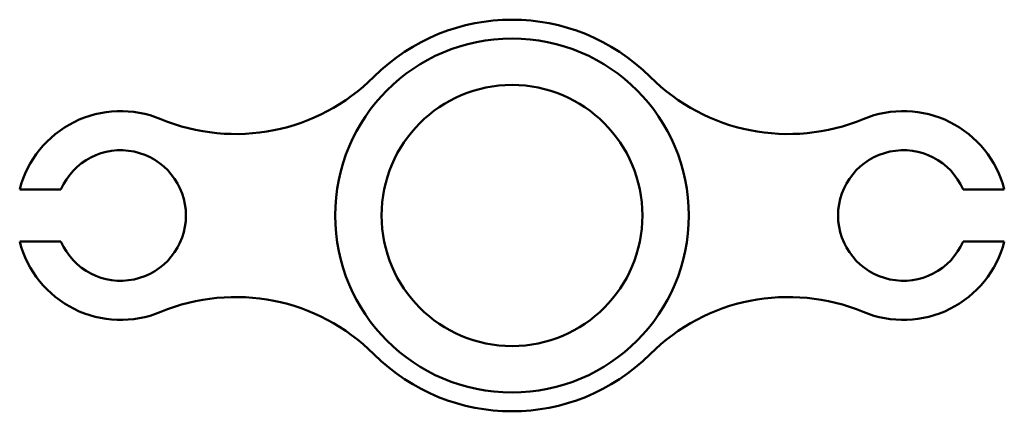
# Model space of a CAD drawing. Units: inches. Extents: x -84 to 294, y 266 to 416.
import ezdxf

# ---------------------------------------------------------------- set-up
doc = ezdxf.new("R2010")
doc.units = ezdxf.units.IN
doc.header["$MEASUREMENT"] = 0
doc.layers.add('M-OUTL', color=7, linetype='Continuous', lineweight=50)

msp = doc.modelspace()

# ---------------------------------------------------------------- linework, layer by layer
at = {"layer": 'M-OUTL'}
for p, q in [((-67.96, 350.79, 10), (-83.78, 350.79, 10)), ((277.86, 350.79, 10), (293.68, 350.79, 10)), ((-67.96, 330.79, 10), (-83.78, 330.79, 10)), ((277.86, 330.79, 10), (293.68, 330.79, 10))]:
    msp.add_line(p, q, dxfattribs=at)
for centre, radius in [((104.95, 340.79, 30), 67.8), ((104.95, 340.79, 20), 50)]:
    msp.add_circle(centre, radius, dxfattribs=at)
for centre, radius, start, end in [((104.95, 340.79, 10), 75, 45.0806, 134.9194), ((-0.97, 447, 10), 75, 247.4597, 314.9194), ((210.86, 447, 10), 75, 225.0806, 292.5403), ((-45.05, 340.79, 10), 40, 67.4597, 165.5225), ((254.95, 340.79, 10), 40, 14.4775, 112.5403), ((-45.05, 340.79, 10), 25, 203.5782, 156.4218), ((254.95, 340.79, 10), 25, 23.5782, 336.4218), ((-45.05, 340.79, 10), 40, 194.4775, 292.5403), ((254.95, 340.79, 10), 40, 247.4597, 345.5225), ((-0.97, 234.57, 10), 75, 45.0806, 112.5403), ((210.86, 234.57, 10), 75, 67.4597, 134.9194), ((104.95, 340.79, 10), 75, 225.0806, 314.9194)]:
    msp.add_arc(centre, radius, start, end, dxfattribs=at)

doc.saveas('drawing.dxf')
